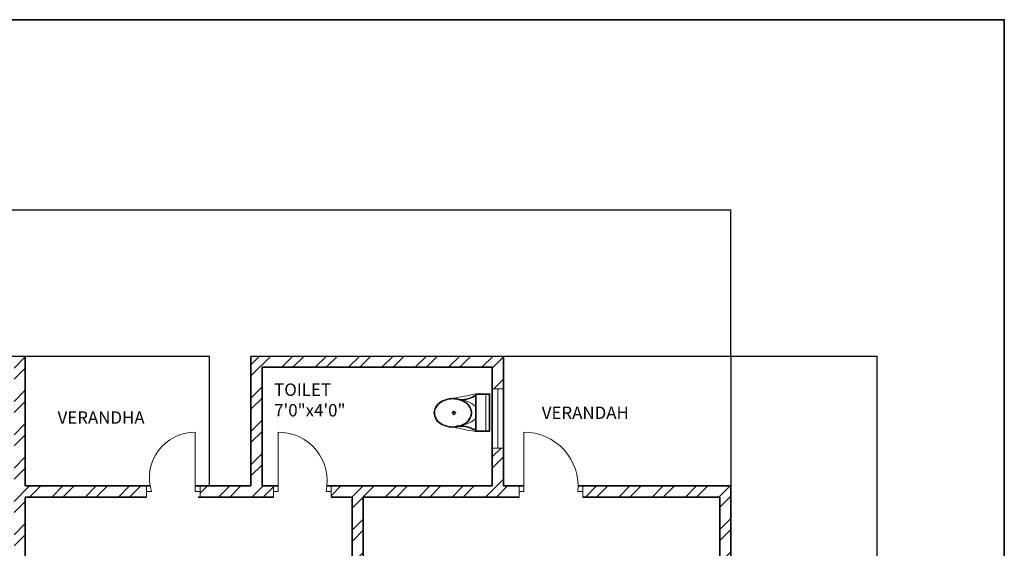
# Model space of a CAD drawing. Units: inches. Extents: x 1962 to 2771, y 1245 to 2660.
# Tile 114 of 114: x 2374 to 2771, y 2447 to 2660. Entities that reach past the tile are written whole.
import ezdxf

# ---------------------------------------------------------------- set-up
doc = ezdxf.new("R2010")
doc.units = ezdxf.units.IN
for name, color, linetype, lineweight in [('A-ANNO-DIMS', 2, 'Continuous', 18), ('A-ANNO-TTLB', 7, 'Continuous', 35), ('A-AREA-IDEN', 7, 'Continuous', 18), ('A-DOOR', 3, 'Continuous', 18), ('A-FLOR-BALC', 7, 'Continuous', 25), ('A-FLOR-FIXT', 8, 'Continuous', 18), ('A-GLAZ', 4, 'Continuous', 18), ('A-WALL', 7, 'Continuous', 35), ('A-WALL-PATT', 252, 'Continuous', 13)]:
    doc.layers.add(name, color=color, linetype=linetype, lineweight=lineweight)
doc.styles.get("Standard").update_dxf_attribs({"font": 'arial.ttf'})
doc.dimstyles.get("Standard").update_dxf_attribs({"dimtxt": 0.18, "dimasz": 0.18, "dimexe": 0.18, "dimexo": 0.0625, "dimgap": 0.09, "dimtad": 0, "dimtih": 1, "dimtoh": 1, "dimdec": 4, "dimzin": 0, "dimdsep": 46, "dimtxsty": 'Standard', "dimcen": 0.09, "dimadec": 0, "dimazin": 0, "dimtfac": 1, "dimtdec": 4, "dimtofl": 0, "dimtmove": 0, "dimatfit": 3, "dimfxl": 1, "dimtolj": 1, "dimtzin": 0, "dimarcsym": 0})

# ---------------------------------------------------------------- blocks, each defined once
blk = doc.blocks.new('A$C31115884')
for p, q in [((283, 498), (223, 498)), ((258, 466), (258, 523)), ((0, 200), (0, 0)), ((520, 200), (0, 200)), ((10, 190), (10, 10)), ((510, 190), (10, 190)), ((510, 10), (510, 190)), ((520, 0), (520, 200)), ((510, 54), (0, 54)), ((10, 10), (510, 10)), ((0, 0), (520, 0))]:
    blk.add_line(p, q)
blk.add_circle((256, 496), 23.6)
for centre, radius, start, end in [((2778, -205), 2807, 165.4549, 171.7133), ((-295, 403), 365, 324.2091, 9.3499), ((-295, 403), 375, 324.2091, 9.3499), ((139, 406), 293, 315.8436, 2.6563), ((806, 403), 375, 179.2036, 215.7909), ((806, 403), 365, 170.6501, 215.7909), ((3237, 905), 2807, 188.2867, 194.5451), ((384, 406), 293, 190.2774, 224.1564)]:
    blk.add_arc(centre, radius, start, end)
blk.add_ellipse((256, 510), major_axis=(0, -261), ratio=0.772727)
blk.add_open_spline([(256, 259), (263, 259), (270, 260), (288, 262), (299, 265), (320, 273), (330, 278), (350, 291), (360, 299), (378, 316), (386, 326), (402, 347), (409, 358), (421, 383), (427, 395), (436, 422), (440, 436), (445, 465), (447, 480), (448, 509), (448, 524), (445, 553), (443, 568), (436, 596), (432, 610), (422, 636), (416, 649), (402, 672), (395, 683), (379, 703), (370, 712), (351, 728), (341, 735), (321, 746), (310, 751), (289, 757), (278, 759), (256, 761), (245, 761), (223, 757), (212, 754), (191, 746), (181, 741), (161, 728), (151, 720), (133, 703), (125, 693), (110, 672), (103, 660), (90, 636), (85, 623), (76, 596), (72, 582), (67, 553), (66, 538), (64, 509), (65, 494), (68, 465), (70, 450), (77, 422), (81, 408), (91, 382), (97, 370), (111, 346), (118, 335), (135, 316), (144, 307), (162, 291), (172, 284), (193, 273), (203, 269), (225, 262), (236, 260), (250, 259), (253, 259), (256, 259)], degree=3, knots=[0, 0, 0, 0, 0.110105, 0.110105, 0.285049, 0.285049, 0.459994, 0.459994, 0.634938, 0.634938, 0.809882, 0.809882, 0.984827, 0.984827, 1.159771, 1.159771, 1.334715, 1.334715, 1.50966, 1.50966, 1.684604, 1.684604, 1.859549, 1.859549, 2.034493, 2.034493, 2.209437, 2.209437, 2.384382, 2.384382, 2.559326, 2.559326, 2.73427, 2.73427, 2.909215, 2.909215, 3.084159, 3.084159, 3.259103, 3.259103, 3.434048, 3.434048, 3.608992, 3.608992, 3.783936, 3.783936, 3.958881, 3.958881, 4.133825, 4.133825, 4.30877, 4.30877, 4.483714, 4.483714, 4.658658, 4.658658, 4.833603, 4.833603, 5.008547, 5.008547, 5.183491, 5.183491, 5.358436, 5.358436, 5.53338, 5.53338, 5.708324, 5.708324, 5.883269, 5.883269, 6.058213, 6.058213, 6.233158, 6.233158, 6.283185, 6.283185, 6.283185, 6.283185])
blk = doc.blocks.new('WIN-24IN-A')
for p, q in [((0, 24), (4.5, 24)), ((4.5, 24), (2.25, 24)), ((2.25, 24), (2.25, 0)), ((2.25, 0), (0, 0)), ((0, 0), (4.5, 0))]:
    blk.add_line(p, q)
blk = doc.blocks.new('*D40')
at = {"layer": 'A-ANNO-DIMS', "color": 0, "lineweight": -2, "transparency": 16777216}
for p, q in [((2072.02, 2033.91), (2072.02, 2583.47)), ((2072.2, 2583.29), (2366.02, 2583.29)), ((2660.63, 2583.29), (2366.81, 2583.29)), ((2660.81, 2524.41), (2660.81, 2583.47))]:
    blk.add_line(p, q, dxfattribs=at)
at = {"layer": 'A-ANNO-DIMS', "color": 0, "transparency": 16777216}
for points in [[(2072.2, 2583.32), (2072.2, 2583.26), (2072.02, 2583.29)], [(2660.63, 2583.32), (2660.63, 2583.26), (2660.81, 2583.29)]]:
    blk.add_solid(points, dxfattribs=at)
at = {"layer": 'Defpoints', "color": 0, "transparency": 16777216}
for p in [(2660.81, 2583.29), (2660.81, 2524.34), (2072.02, 2033.84)]:
    blk.add_point(p, dxfattribs=at)
at = {"layer": 'A-ANNO-DIMS', "color": 0, "transparency": 16777216, "insert": (2366.41, 2583.29), "char_height": 0.18, "attachment_point": 5}
blk.add_mtext('\\A1;588.8', dxfattribs=at)
blk = doc.blocks.new('*D42')
at = {"layer": 'A-ANNO-DIMS', "color": 0, "lineweight": -2, "transparency": 16777216}
for p, q in [((2660.87, 2524.34), (2719.94, 2524.34)), ((2719.76, 2524.16), (2719.76, 1979.28)), ((2719.76, 1434.02), (2719.76, 1978.91)), ((2660.87, 1433.84), (2719.94, 1433.84))]:
    blk.add_line(p, q, dxfattribs=at)
at = {"layer": 'A-ANNO-DIMS', "color": 0, "transparency": 16777216}
for points in [[(2719.73, 2524.16), (2719.79, 2524.16), (2719.76, 2524.34)], [(2719.73, 1434.02), (2719.79, 1434.02), (2719.76, 1433.84)]]:
    blk.add_solid(points, dxfattribs=at)
at = {"layer": 'Defpoints', "color": 0, "transparency": 16777216}
for p in [(2660.81, 2524.34), (2719.76, 2524.34), (2660.81, 1433.84)]:
    blk.add_point(p, dxfattribs=at)
at = {"layer": 'A-ANNO-DIMS', "color": 0, "transparency": 16777216, "insert": (2719.76, 1979.09), "char_height": 0.18, "attachment_point": 5}
blk.add_mtext('\\A1;1090.5', dxfattribs=at)

msp = doc.modelspace()

# ---------------------------------------------------------------- hatches: boundary and pattern name
at = {"layer": 'A-WALL-PATT'}
h = msp.add_hatch(dxfattribs=at)
h.set_pattern_fill('ANSI32', color=256)
h.paths.add_polyline_path([(2090.8074, 2467.3437), (2141.6481, 2467.3437), (2141.6481, 2469.5937), (2141.6481, 2471.8437), (2086.3074, 2471.8437), (2086.3074, 2422.5333), (2090.8074, 2422.5333)])
h.paths.add_polyline_path([(2282.7664, 2471.8437), (2204.8982, 2471.8437), (2204.8982, 2467.3437), (2234.8074, 2467.3437), (2234.8074, 2311.3437), (2228.7492, 2311.3437), (2228.7492, 2306.8437), (2234.8074, 2306.8437), (2331.9227, 2306.8437), (2331.9227, 2309.0937), (2331.9227, 2311.3437), (2239.3074, 2311.3437), (2239.3074, 2467.3437), (2282.7664, 2467.3437), (2282.7664, 2469.5937)])
h.paths.add_polyline_path([(2471.4531, 2519.8437), (2552.011, 2519.8437), (2564.3996, 2519.8437), (2564.3996, 2511.1389), (2568.8996, 2511.1389), (2568.8996, 2524.3437), (2466.9531, 2524.3437), (2466.9531, 2471.8437), (2450.0749, 2471.8437), (2446.4672, 2471.8437), (2446.4672, 2467.3437), (2450.0749, 2467.3437), (2475.9988, 2467.3437), (2475.9988, 2469.5937), (2475.9988, 2471.8437), (2471.4531, 2471.8437)])
h.paths.add_polyline_path([(2575.2231, 2469.5937), (2575.2231, 2471.8437), (2568.8996, 2471.8437), (2568.8996, 2487.1389), (2564.3996, 2487.1389), (2564.3996, 2471.8437), (2556.511, 2471.8437), (2499.2904, 2471.8437), (2499.2904, 2467.3437), (2507.8074, 2467.3437), (2507.8074, 2311.3437), (2414.863, 2311.3437), (2414.863, 2306.8437), (2512.3074, 2306.8437), (2517.0114, 2306.8437), (2517.0114, 2309.0937), (2517.0114, 2311.3437), (2512.3074, 2311.3437), (2512.3074, 2467.3437), (2575.2231, 2467.3437)])
h.paths.add_polyline_path([(2660.8074, 2471.8437), (2600.9602, 2471.8437), (2600.9602, 2467.3437), (2656.3074, 2467.3437), (2656.3074, 2432.5704), (2660.8074, 2432.5704)])
h.paths.add_polyline_path([(2660.8074, 2372.5704), (2656.3074, 2372.5704), (2656.3074, 2311.3437), (2600.276, 2311.3437), (2600.276, 2309.0937), (2600.276, 2306.8437), (2656.3074, 2306.8437), (2656.3074, 2296.2593), (2660.8074, 2296.2593)])
h.paths.add_polyline_path([(2572.3074, 2306.8437), (2577.1385, 2306.8437), (2577.1385, 2311.3437), (2551.082, 2311.3437), (2551.082, 2306.8437), (2567.8074, 2306.8437), (2567.8074, 2258.8437), (2540.0574, 2258.8437), (2540.0574, 2256.5937), (2540.0574, 2254.3437), (2567.8074, 2254.3437), (2656.3074, 2254.3437), (2656.3074, 2236.9085), (2660.8074, 2236.9085), (2660.8074, 2272.2593), (2656.3074, 2272.2593), (2656.3074, 2258.8437), (2572.3074, 2258.8437)])
h.paths.add_polyline_path([(2512.3074, 2254.3437), (2518.8716, 2254.3437), (2518.8716, 2256.5937), (2518.8716, 2258.8437), (2507.8074, 2258.8437), (2507.8074, 2177.8437), (2567.8074, 2177.8437), (2567.8074, 2172.9628), (2572.3074, 2172.9628), (2572.3074, 2177.8437), (2656.3074, 2177.8437), (2656.3074, 2166.4846), (2660.8074, 2166.4846), (2660.8074, 2200.9085), (2656.3074, 2200.9085), (2656.3074, 2182.3437), (2512.3074, 2182.3437)])
h.paths.add_polyline_path([(2656.3074, 2129.8437), (2572.3074, 2129.8437), (2572.3074, 2150.3044), (2570.0574, 2150.3044), (2567.8074, 2150.3044), (2567.8074, 2129.8437), (2507.8074, 2129.8437), (2507.8074, 2116.3027), (2510.0574, 2116.3027), (2512.3074, 2116.3027), (2512.3074, 2125.3437), (2567.8074, 2125.3437), (2572.3074, 2125.3437), (2656.3074, 2125.3437)])
h.paths.add_polyline_path([(2090.8074, 2362.5333), (2086.3074, 2362.5333), (2086.3074, 2298.6242), (2090.8074, 2298.6242), (2090.8074, 2306.8437), (2174.8074, 2306.8437), (2174.8074, 2286.4178), (2179.3074, 2286.4178), (2179.3074, 2306.8437), (2192.8641, 2306.8437), (2192.8641, 2309.0937), (2192.8641, 2311.3437), (2090.8074, 2311.3437)])
h.paths.add_polyline_path([(2209.156, 2258.8437), (2179.3074, 2258.8437), (2179.3074, 2263.2236), (2177.0574, 2263.2236), (2174.8074, 2263.2236), (2174.8074, 2258.8437), (2090.8074, 2258.8437), (2090.8074, 2274.6242), (2086.3074, 2274.6242), (2086.3074, 2238.2967), (2088.5574, 2238.2967), (2090.8074, 2238.2967), (2090.8074, 2254.3437), (2209.156, 2254.3437)])
h.paths.add_polyline_path([(2090.8074, 2177.8437), (2234.8074, 2177.8437), (2234.8074, 2173.1428), (2239.3074, 2173.1428), (2239.3074, 2258.8437), (2230.8442, 2258.8437), (2230.8442, 2256.5937), (2230.8442, 2254.3437), (2234.8074, 2254.3437), (2234.8074, 2182.3437), (2090.8074, 2182.3437), (2090.8074, 2202.2967), (2086.3074, 2202.2967), (2086.3074, 2140.0389), (2090.8074, 2140.0389)])
h.paths.add_polyline_path([(2090.8074, 2080.0389), (2086.3074, 2080.0389), (2086.3074, 2033.8437), (2090.8074, 2033.8437)], flags=17)
h.paths.add_polyline_path([(2244.9405, 2033.8437), (2239.3074, 2033.8437), (2239.3074, 2142.0665), (2237.2592, 2142.0665), (2234.8074, 2142.0665), (2234.8074, 2033.8437), (2090.8074, 2033.8437), (2076.5204, 2033.8437), (2072.0204, 2033.8437), (2072.0204, 2000.4493), (2076.5204, 2000.4493), (2076.5204, 2029.3437), (2090.8074, 2029.3437), (2244.9405, 2029.3437), (2244.9405, 2031.5937)])
h.paths.add_polyline_path([(2234.8074, 1933.3437), (2076.5204, 1933.3437), (2076.5204, 1952.4493), (2074.2704, 1952.4493), (2072.0204, 1952.4493), (2072.0204, 1933.3437), (2072.0204, 1928.8437), (2234.8074, 1928.8437)])
h.paths.add_polyline_path([(2090.8074, 1928.8437), (2086.3074, 1928.8437), (2086.3074, 1906.5013), (2090.8074, 1906.5013)])
h.paths.add_polyline_path([(2090.8074, 1846.5013), (2086.3074, 1846.5013), (2086.3074, 1769.9917), (2088.5574, 1769.9917), (2090.8074, 1769.9917), (2090.8074, 1780.3437), (2234.8074, 1780.3437), (2234.8074, 1708.3437), (2230.3764, 1708.3437), (2230.3764, 1703.8437), (2239.3074, 1703.8437), (2239.3074, 1792.6669), (2237.0574, 1792.6669), (2234.8074, 1792.6669), (2234.8074, 1784.8437), (2090.8074, 1784.8437)])
h.paths.add_polyline_path([(2239.3074, 1928.8437), (2244.9405, 1928.8437), (2244.9405, 1931.0937), (2244.9405, 1933.3437), (2234.8074, 1933.3437), (2234.8074, 1928.8437), (2234.8074, 1825.5949), (2239.3074, 1825.5949)])
h.paths.add_polyline_path([(2148.0425, 1649.0937), (2148.0425, 1651.3437), (2090.8074, 1651.3437), (2090.8074, 1646.8437), (2148.0425, 1646.8437)], flags=0)
h.paths.add_polyline_path([(2207.5601, 1708.3437), (2090.8074, 1708.3437), (2090.8074, 1703.8437), (2174.8074, 1703.8437), (2174.8074, 1651.3437), (2170.4457, 1651.3437), (2170.4457, 1646.8437), (2195.9924, 1646.8437), (2195.9924, 1649.0937), (2195.9924, 1651.3437), (2179.3074, 1651.3437), (2179.3074, 1703.8437), (2207.5601, 1703.8437), (2207.5601, 1706.0937)])
h.paths.add_polyline_path([(2090.8074, 1733.9917), (2086.3074, 1733.9917), (2086.3074, 1696.1032), (2088.5574, 1696.1032), (2090.8074, 1696.1032)])
h.paths.add_polyline_path([(2090.8074, 1672.1032), (2086.3074, 1672.1032), (2086.3074, 1600.3335), (2090.8074, 1600.3335)])
h.paths.add_polyline_path([(2090.8074, 1540.3335), (2086.3074, 1540.3335), (2086.3074, 1486.3437), (2139.6766, 1486.3437), (2139.6766, 1490.8437), (2090.8074, 1490.8437)])
h.paths.add_polyline_path([(2302.3876, 1490.8437), (2239.3074, 1490.8437), (2239.3074, 1646.8437), (2335.9994, 1646.8437), (2335.9994, 1651.3437), (2229.884, 1651.3437), (2229.884, 1646.8437), (2234.8074, 1646.8437), (2234.8074, 1490.8437), (2202.7103, 1490.8437), (2202.7103, 1488.5937), (2202.7103, 1486.3437), (2275.0699, 1486.3437), (2275.0699, 1475.772), (2279.5699, 1475.772), (2279.5699, 1486.3437), (2302.3876, 1486.3437)])
h.paths.add_polyline_path([(2279.5699, 1451.772), (2275.0699, 1451.772), (2275.0699, 1438.3437), (2174.8074, 1438.3437), (2174.8074, 1486.3437), (2179.7922, 1486.3437), (2179.7922, 1490.8437), (2163.3585, 1490.8437), (2163.3585, 1488.5937), (2163.3585, 1486.3437), (2170.3074, 1486.3437), (2170.3074, 1433.8437), (2279.5699, 1433.8437)])
h.paths.add_polyline_path([(2427.2363, 1490.8437), (2375.8074, 1490.8437), (2375.8074, 1646.8437), (2381.6401, 1646.8437), (2381.6401, 1651.3437), (2365.887, 1651.3437), (2365.887, 1649.0937), (2365.887, 1646.8437), (2371.3074, 1646.8437), (2371.3074, 1490.8437), (2327.5627, 1490.8437), (2327.5627, 1488.5937), (2327.5627, 1486.3437), (2371.3074, 1486.3437), (2371.3074, 1433.8437), (2375.8074, 1433.8437), (2375.8074, 1486.3437), (2427.2363, 1486.3437)])
h.paths.add_polyline_path([(2512.3074, 1646.8437), (2519.4351, 1646.8437), (2519.4351, 1649.0937), (2519.4351, 1651.3437), (2507.8074, 1651.3437), (2416.0063, 1651.3437), (2416.0063, 1649.0937), (2416.0063, 1646.8437), (2507.8074, 1646.8437), (2507.8074, 1490.8437), (2497.0532, 1490.8437), (2497.0532, 1488.5937), (2497.0532, 1486.3437), (2574.9344, 1486.3437), (2574.9344, 1476.0181), (2579.4344, 1476.0181), (2579.4344, 1486.3437), (2584.4872, 1486.3437), (2584.3074, 1490.8437), (2512.3074, 1490.8437)])
h.paths.add_polyline_path([(2470.5091, 1486.3437), (2473.9767, 1486.3437), (2473.9767, 1490.8437), (2449.6605, 1490.8437), (2449.6605, 1488.5937), (2449.6605, 1486.3437), (2466.0091, 1486.3437), (2466.0091, 1433.8437), (2470.5091, 1433.8437), (2579.4344, 1433.8437), (2579.4344, 1452.0181), (2574.9344, 1452.0181), (2574.9344, 1438.3437), (2554.5091, 1438.3437), (2470.5091, 1438.3437)])
h.paths.add_polyline_path([(2656.3074, 1490.8437), (2611.86, 1490.8437), (2611.86, 1486.3437), (2656.3074, 1486.3437)])
h.paths.add_polyline_path([(2660.8074, 1532.7007), (2658.5574, 1532.7007), (2656.3074, 1532.7007), (2656.3074, 1486.3437), (2660.8074, 1486.3437)])
h.paths.add_polyline_path([(2660.8074, 1664.9663), (2656.3074, 1664.9663), (2656.3074, 1651.3437), (2602.2313, 1651.3437), (2602.2313, 1646.8437), (2656.3074, 1646.8437), (2656.3074, 1592.7007), (2660.8074, 1592.7007)])
h.paths.add_polyline_path([(2660.8074, 1724.5221), (2656.3074, 1724.5221), (2656.3074, 1703.8437), (2542.4725, 1703.8437), (2542.4725, 1699.3437), (2567.8074, 1699.3437), (2567.8074, 1651.3437), (2552.7766, 1651.3437), (2552.7766, 1649.0937), (2552.7766, 1646.8437), (2577.2878, 1646.8437), (2577.2878, 1649.0937), (2577.2878, 1651.3437), (2572.3074, 1651.3437), (2572.3074, 1699.3437), (2656.3074, 1699.3437), (2656.3074, 1688.9663), (2660.8074, 1688.9663)])
h.paths.add_polyline_path([(2660.8074, 1880.6524), (2656.3074, 1880.6524), (2656.3074, 1832.8437), (2512.3074, 1832.8437), (2512.3074, 1837.8959), (2507.8074, 1837.8959), (2507.8074, 1828.3437), (2567.8074, 1828.3437), (2567.8074, 1804.3437), (2572.3074, 1804.3437), (2572.3074, 1828.3437), (2656.3074, 1828.3437), (2656.3074, 1818.6778), (2660.8074, 1818.6778)])
h.paths.add_polyline_path([(2660.8074, 1794.6778), (2656.3074, 1794.6778), (2656.3074, 1780.3437), (2572.3074, 1780.3437), (2572.3074, 1783.0303), (2570.0574, 1783.0303), (2567.8074, 1783.0303), (2567.8074, 1780.3437), (2507.8074, 1780.3437), (2507.8074, 1699.3437), (2517.8858, 1699.3437), (2517.8858, 1701.5937), (2517.8858, 1703.8437), (2512.3074, 1703.8437), (2512.3074, 1775.8437), (2656.3074, 1775.8437), (2656.3074, 1760.5221), (2660.8074, 1760.5221)])
h.paths.add_polyline_path([(2660.8074, 1981.3437), (2660.8074, 2020.2808), (2658.5574, 2020.2808), (2656.3074, 2020.2808), (2656.3074, 1981.3437), (2512.3074, 1981.3437), (2512.3074, 2086.6996), (2507.8074, 2086.6996), (2507.8074, 1981.3437), (2375.8074, 1981.3437), (2375.8074, 1986.8505), (2373.5574, 1986.8505), (2371.3074, 1986.8505), (2371.3074, 1973.2607), (2375.8074, 1973.2607), (2375.8074, 1976.8437), (2507.8074, 1976.8437), (2507.8074, 1865.4281), (2510.0574, 1865.4281), (2512.3074, 1865.4281), (2512.3074, 1976.8437), (2660.8074, 1976.8437)])
h.paths.add_polyline_path([(2375.8074, 1940.297), (2373.5574, 1940.297), (2371.3074, 1940.297), (2371.3074, 1933.3437), (2278.4434, 1933.3437), (2278.4434, 1928.8437), (2371.3074, 1928.8437), (2371.3074, 1651.3437), (2375.8074, 1651.3437)])
h.paths.add_polyline_path([(2660.8074, 1976.8437), (2656.3074, 1976.8437), (2656.3074, 1940.6524), (2660.8074, 1940.6524)], flags=17)
h.paths.add_polyline_path([(2660.8074, 2142.4846), (2656.3074, 2142.4846), (2656.3074, 2080.2808), (2660.8074, 2080.2808)])
h.paths.add_polyline_path([(2381.4189, 2311.3437), (2375.8074, 2311.3437), (2375.8074, 2467.3437), (2424.7242, 2467.3437), (2424.7242, 2469.5937), (2424.7242, 2471.8437), (2375.8074, 2471.8437), (2375.8074, 2524.3437), (2371.3074, 2524.3437), (2371.3074, 2471.8437), (2307.2097, 2471.8437), (2307.2097, 2467.3437), (2371.3074, 2467.3437), (2371.3074, 2311.3437), (2366.8901, 2311.3437), (2366.8901, 2306.8437), (2371.3074, 2306.8437), (2371.3074, 2033.8437), (2279.6589, 2033.8437), (2279.6589, 2029.3437), (2371.3074, 2029.3437), (2371.3074, 2014.2598), (2375.8074, 2014.2598), (2375.8074, 2306.8437), (2381.4189, 2306.8437)])
h.paths.add_polyline_path([(2263.3074, 2524.3437), (2170.3074, 2524.3437), (2170.3074, 2519.8437), (2170.3074, 2471.8437), (2165.0312, 2471.8437), (2165.0312, 2467.3437), (2179.6721, 2467.3437), (2179.6721, 2469.5161), (2179.6721, 2471.8437), (2174.8074, 2471.8437), (2174.8074, 2519.8437), (2258.8074, 2519.8437), (2258.8074, 2511.6436), (2263.3074, 2511.6436)])
h.paths.add_polyline_path([(2245.0232, 1361.4123), (2492.9468, 1361.4123), (2492.9468, 1398.505), (2245.0232, 1398.505)], flags=9)
h.paths.add_polyline_path([(2388.1434, 2086.6936), (2425.0704, 2086.6936), (2425.0704, 2105.3509), (2388.1434, 2105.3509)], flags=9)
h.paths.add_polyline_path([(2404.922, 2242.6744), (2445.7337, 2242.6744), (2445.7337, 2261.3318), (2404.922, 2261.3318)], flags=9)
h.paths.add_polyline_path([(2269.4107, 2156.7935), (2306.3378, 2156.7935), (2306.3378, 2175.4508), (2269.4107, 2175.4508)], flags=9)
h.paths.add_polyline_path([(2269.3277, 2233.4343), (2306.2547, 2233.4343), (2306.2547, 2252.0917), (2269.3277, 2252.0917)], flags=9)
h.paths.add_polyline_path([(2431.6052, 2320.6922), (2470.4456, 2320.6922), (2470.4456, 2339.3495), (2431.6052, 2339.3495)], flags=25)
h.paths.add_polyline_path([(2249.6902, 2315.7608), (2288.5306, 2315.7608), (2288.5306, 2334.4182), (2249.6902, 2334.4182)], flags=25)
h.paths.add_polyline_path([(2096.9301, 2314.3181), (2135.7704, 2314.3181), (2135.7704, 2332.9755), (2096.9301, 2332.9755)], flags=25)
h.paths.add_polyline_path([(2134.3475, 2285.7089), (2161.4655, 2285.7089), (2161.4655, 2304.3662), (2134.3475, 2304.3662)], flags=9)
h.paths.add_polyline_path([(2126.5155, 2209.4076), (2159.9227, 2209.4076), (2159.9227, 2228.065), (2126.5155, 2228.065)], flags=25)
h.paths.add_polyline_path([(2110.5753, 2141.5299), (2149.4157, 2141.5299), (2149.4157, 2160.1872), (2110.5753, 2160.1872)], flags=25)
h.paths.add_polyline_path([(2249.8618, 1968.3317), (2286.3966, 1968.3317), (2286.3966, 1986.989), (2249.8618, 1986.989)], flags=9)
h.paths.add_polyline_path([(2395.9507, 1777.0051), (2436.7624, 1777.0051), (2436.7624, 1795.6625), (2395.9507, 1795.6625)], flags=9)
h.paths.add_polyline_path([(2398.5259, 1888.5651), (2435.0062, 1888.5651), (2435.0062, 1907.2224), (2398.5259, 1907.2224)], flags=25)
h.paths.add_polyline_path([(2259.3506, 1728.3559), (2296.2776, 1728.3559), (2296.2776, 1747.0132), (2259.3506, 1747.0132)], flags=9)
h.paths.add_polyline_path([(2271.3698, 1845.268), (2308.2968, 1845.268), (2308.2968, 1863.9253), (2271.3698, 1863.9253)], flags=9)
h.paths.add_polyline_path([(2120.9355, 1786.3027), (2159.7759, 1786.3027), (2159.7759, 1804.9601), (2120.9355, 1804.9601)], flags=25)
h.paths.add_polyline_path([(2121.3164, 1732.1043), (2154.7236, 1732.1043), (2154.7236, 1750.7616), (2121.3164, 1750.7616)], flags=25)
h.paths.add_polyline_path([(2118.3706, 1678.8997), (2147.5282, 1678.8997), (2147.5282, 1697.557), (2118.3706, 1697.557)], flags=25)
h.paths.add_polyline_path([(2385.9227, 1493.557), (2424.763, 1493.557), (2424.763, 1512.2143), (2385.9227, 1512.2143)], flags=25)
h.paths.add_polyline_path([(2248.7058, 1500.0256), (2287.5462, 1500.0256), (2287.5462, 1518.6829), (2248.7058, 1518.6829)], flags=25)
h.paths.add_polyline_path([(2104.1669, 1617.3771), (2143.0073, 1617.3771), (2143.0073, 1636.0344), (2104.1669, 1636.0344)], flags=9)
h.paths.add_polyline_path([(2096.0714, 1447.8824), (2137.3845, 1447.8824), (2137.3845, 1458.1859), (2096.0714, 1458.1859)], flags=9)
h.paths.add_polyline_path([(2180.6114, 1440.325), (2209.7689, 1440.325), (2209.7689, 1458.9823), (2180.6114, 1458.9823)], flags=25)
h.paths.add_polyline_path([(2316.1698, 1447.9637), (2357.4829, 1447.9637), (2357.4829, 1458.2673), (2316.1698, 1458.2673)], flags=9)
h.paths.add_polyline_path([(2397.6187, 1447.9637), (2438.9318, 1447.9637), (2438.9318, 1458.2673), (2397.6187, 1458.2673)], flags=9)
h.paths.add_polyline_path([(2473.0778, 1439.5953), (2502.2354, 1439.5953), (2502.2354, 1458.2527), (2473.0778, 1458.2527)], flags=25)
h.paths.add_polyline_path([(2589.7027, 1447.8819), (2631.0158, 1447.8819), (2631.0158, 1458.1855), (2589.7027, 1458.1855)], flags=9)
h.paths.add_polyline_path([(2522.4009, 1497.5285), (2561.2413, 1497.5285), (2561.2413, 1516.1859), (2522.4009, 1516.1859)], flags=25)
h.paths.add_polyline_path([(2579.6565, 1671.3482), (2608.8141, 1671.3482), (2608.8141, 1690.0056), (2579.6565, 1690.0056)], flags=25)
h.paths.add_polyline_path([(2544.7038, 1725.5064), (2578.1111, 1725.5064), (2578.1111, 1744.1637), (2544.7038, 1744.1637)], flags=25)
h.paths.add_polyline_path([(2578.1191, 1807.472), (2607.2766, 1807.472), (2607.2766, 1826.1293), (2578.1191, 1826.1293)], flags=25)
h.paths.add_polyline_path([(2595.0614, 1835.1839), (2633.9018, 1835.1839), (2633.9018, 1853.8413), (2595.0614, 1853.8413)], flags=25)
h.paths.add_polyline_path([(2567.0097, 2097.7035), (2605.8501, 2097.7035), (2605.8501, 2116.3609), (2567.0097, 2116.3609)], flags=9)
h.paths.add_polyline_path([(2586.644, 2134.6454), (2615.8015, 2134.6454), (2615.8015, 2153.3027), (2586.644, 2153.3027)], flags=9)
h.paths.add_polyline_path([(2544.6185, 2212.6783), (2578.0258, 2212.6783), (2578.0258, 2231.3356), (2544.6185, 2231.3356)], flags=25)
h.paths.add_polyline_path([(2577.0273, 2256.9023), (2606.1849, 2256.9023), (2606.1849, 2275.5597), (2577.0273, 2275.5597)], flags=24)
h.paths.add_polyline_path([(2605.2683, 2315.2821), (2644.1087, 2315.2821), (2644.1087, 2333.9395), (2605.2683, 2333.9395)], flags=25)
h.paths.add_polyline_path([(2583.1244, 2496.1815), (2624.4375, 2496.1815), (2624.4375, 2506.4851), (2583.1244, 2506.4851)], flags=9)
h.paths.add_polyline_path([(2474.761, 2497.0823), (2503.9185, 2497.0823), (2503.9185, 2515.7397), (2474.761, 2515.7397)], flags=25)
h.paths.add_polyline_path([(2387.5787, 2494.2563), (2428.902, 2494.2563), (2428.902, 2504.5598), (2387.5787, 2504.5598)], flags=9)
h.paths.add_polyline_path([(2300.1657, 2500.1564), (2341.4788, 2500.1564), (2341.4788, 2510.46), (2300.1657, 2510.46)], flags=25)
h.paths.add_polyline_path([(2176.8589, 2497.5843), (2206.0165, 2497.5843), (2206.0165, 2516.2416), (2176.8589, 2516.2416)], flags=25)
h.paths.add_polyline_path([(2097.4668, 2494.9762), (2138.7799, 2494.9762), (2138.7799, 2505.2798), (2097.4668, 2505.2798)], flags=9)

# ---------------------------------------------------------------- linework, layer by layer
at = {"layer": 'A-ANNO-TTLB'}
msp.add_lwpolyline([(1961.7365, 2660.2579), (2771.213, 2660.2579), (2771.213, 1244.5817), (1961.7365, 1244.5817)], close=True, dxfattribs=at)
at = {"layer": 'A-DOOR'}
for p, q in [((2444.4672, 2469.5937), (2444.4672, 2493.5937)), ((2477.9988, 2469.5937), (2477.9988, 2493.5937)), ((2577.2231, 2469.5937), (2577.2231, 2493.5937)), ((2424.7242, 2471.8437), (2424.7242, 2467.3437)), ((2424.7242, 2467.3437), (2424.7242, 2469.5937)), ((2424.7242, 2469.5937), (2426.7242, 2469.5937)), ((2446.4672, 2469.5937), (2444.4672, 2469.5937)), ((2446.4672, 2471.8437), (2446.4672, 2467.3437)), ((2446.4672, 2467.3437), (2446.4672, 2469.5937)), ((2475.9988, 2471.8437), (2475.9988, 2467.3437)), ((2475.9988, 2467.3437), (2475.9988, 2469.5937)), ((2475.9988, 2469.5937), (2477.9988, 2469.5937)), ((2499.2904, 2469.5937), (2497.2904, 2469.5937)), ((2499.2904, 2471.8437), (2499.2904, 2467.3437)), ((2499.2904, 2467.3437), (2499.2904, 2469.5937)), ((2575.2231, 2471.8437), (2575.2231, 2467.3437)), ((2575.2231, 2467.3437), (2575.2231, 2469.5937)), ((2575.2231, 2469.5937), (2577.2231, 2469.5937)), ((2600.9602, 2469.5937), (2598.9602, 2469.5937)), ((2600.9602, 2471.8437), (2600.9602, 2467.3437)), ((2600.9602, 2467.3437), (2600.9602, 2469.5937))]:
    msp.add_line(p, q, dxfattribs=at)
for centre, radius, start, end in [((2444.4672, 2475.0351), 18.5587, 90, 197.049484), ((2477.9988, 2473.8403), 19.7534, 347.585747, 90), ((2577.2231, 2471.7499), 21.8438, 354.335064, 90)]:
    msp.add_arc(centre, radius, start, end, dxfattribs=at)
at = {"layer": 'A-FLOR-BALC'}
for p, q in [((2277.2053, 2524.3437), (2450.0749, 2524.3437)), ((2375.8074, 2524.3437), (2450.0749, 2524.3437)), ((2450.0749, 2524.3437), (2450.0749, 2471.8437)), ((2450.0749, 2524.3437), (2450.0749, 2519.8437)), ((2466.9531, 2524.3437), (2660.8074, 2524.3437)), ((2660.8074, 2524.3437), (2660.8074, 2471.8437))]:
    msp.add_line(p, q, dxfattribs=at)
at = {"layer": 'A-WALL'}
for p, q in [((2375.8074, 2471.8437), (2375.8074, 2524.3437)), ((2466.9531, 2471.8437), (2466.9531, 2524.3437)), ((2568.8996, 2524.3437), (2568.8996, 2471.8437)), ((2552.011, 2519.8437), (2471.4531, 2519.8437)), ((2471.4531, 2519.8437), (2471.4531, 2471.8437)), ((2564.3996, 2519.8437), (2552.011, 2519.8437)), ((2564.3996, 2471.8437), (2564.3996, 2519.8437)), ((2375.8074, 2471.8437), (2426.1851, 2471.8437)), ((2444.4672, 2471.8437), (2450.0749, 2471.8437)), ((2450.0749, 2471.8437), (2466.9531, 2471.8437)), ((2471.4531, 2471.8437), (2477.9988, 2471.8437)), ((2497.6511, 2471.8437), (2563.4978, 2471.8437)), ((2497.6511, 2471.8437), (2552.011, 2471.8437)), ((2556.511, 2471.8437), (2564.3996, 2471.8437)), ((2568.8996, 2471.8437), (2577.2231, 2471.8437)), ((2599.0667, 2471.8437), (2660.8074, 2471.8437)), ((2660.8074, 2471.8437), (2660.8074, 1976.8437)), ((2375.8074, 2467.3437), (2375.8074, 2311.3437)), ((2375.8074, 2467.3437), (2424.7242, 2467.3437)), ((2450.0749, 2467.3437), (2445.5749, 2467.3437)), ((2446.4672, 2467.3437), (2475.9988, 2467.3437)), ((2499.2904, 2467.3437), (2507.8074, 2467.3437)), ((2507.8074, 2467.3437), (2507.8074, 2311.3437)), ((2512.3074, 2467.3437), (2512.3074, 2311.3437)), ((2512.3074, 2467.3437), (2575.2231, 2467.3437)), ((2567.9978, 2467.3437), (2563.4978, 2467.3437)), ((2600.9602, 2467.3437), (2656.3074, 2467.3437)), ((2656.3074, 2467.3437), (2656.3074, 2311.3437))]:
    msp.add_line(p, q, dxfattribs=at)

# ---------------------------------------------------------------- block references
at = {"layer": 'A-FLOR-FIXT', "xscale": 0.0292470664339069, "yscale": 0.0292470664339069, "zscale": 0.0292470664339069, "rotation": 89.99999999999999}
msp.add_blockref('A$C31115884', (2563.4277, 2493.8843), dxfattribs=at)
at = {"layer": 'A-GLAZ'}
msp.add_blockref('WIN-24IN-A', (2564.3996, 2487.1389), dxfattribs=at)

# ---------------------------------------------------------------- texts
at = {"layer": 'A-AREA-IDEN', "char_height": 5, "attachment_point": 1}
for s, width, insert in [('TOILET\\P7\'0"x4\'0"', 75.707576, (2476.3418, 2513.255)), ('VERANDHA', 121.871813, (2388.8594, 2501.9865)), ('VERANDAH', 93.892548, (2584.4051, 2503.9117))]:
    msp.add_mtext_dynamic_manual_height_columns(s, width=width, gutter_width=12.5, heights=[0], dxfattribs=dict(at, insert=insert))

# ---------------------------------------------------------------- dimensions: what is measured, and where the dimension line sits
at = {"layer": 'A-ANNO-DIMS'}
dim = msp.add_linear_dim(base=(2660.8074, 2583.2937), p1=(2072.0204, 2033.8437), p2=(2660.8074, 2524.3437), dimstyle='Standard', override={"dimdec": 1, "dimlfac": 1, "dimrnd": 0, "dimzin": 0, "dimdsep": 46, "dimlunit": 2}, dxfattribs=at)
dim.commit()
dim.dimension.update_dxf_attribs({"geometry": '*D40', "text_midpoint": (2366.4139, 2583.2937)})
dim = msp.add_linear_dim(base=(2719.7574, 2524.3437), p1=(2660.8074, 1433.8437), p2=(2660.8074, 2524.3437), angle=90, dimstyle='Standard', override={"dimdec": 1, "dimlfac": 1, "dimrnd": 0, "dimzin": 0, "dimdsep": 46, "dimlunit": 2}, dxfattribs=at)
dim.commit()
dim.dimension.update_dxf_attribs({"geometry": '*D42', "text_midpoint": (2719.7574, 1979.0937)})

doc.saveas('drawing.dxf')
